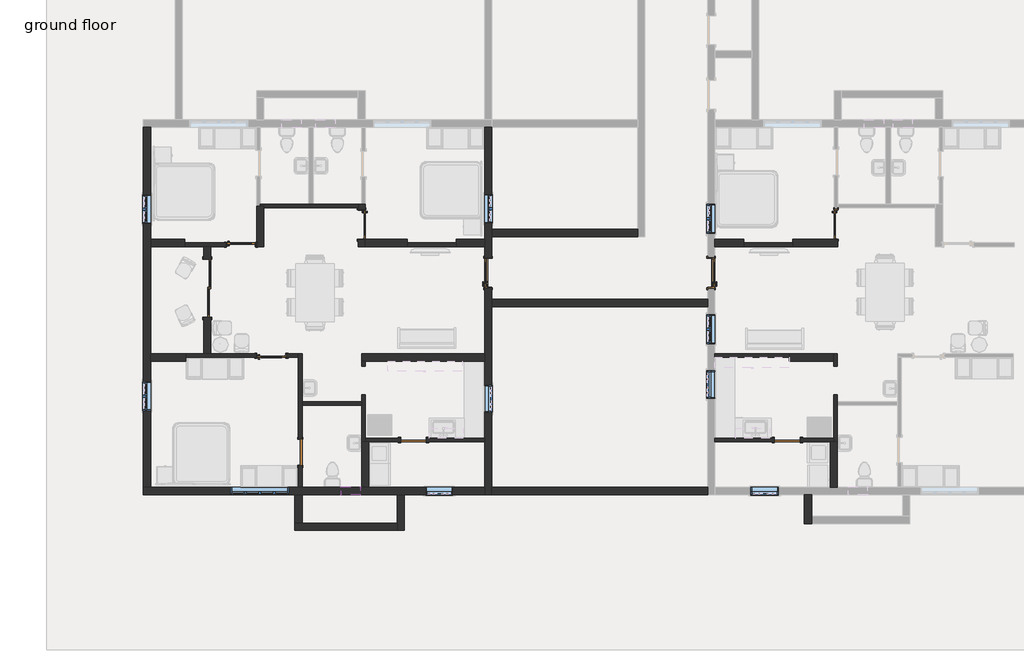
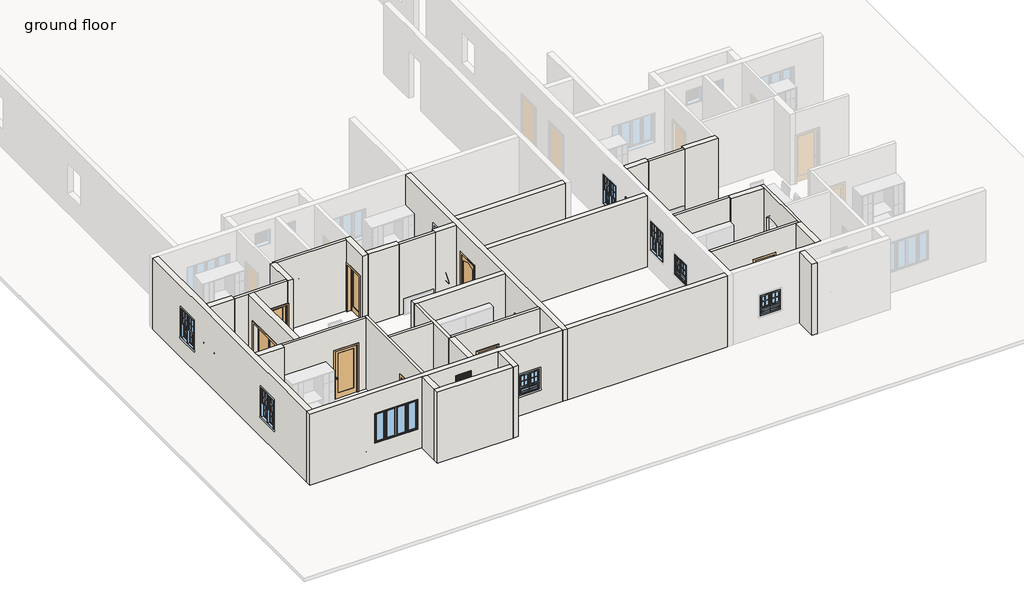
# One storey, part 1 of 16: 35 walls, 11 windows, 10 doors.
"""IFC4 building model written with IfcOpenShell, lengths in millimetres."""

from ifc_helpers import new_model, si_unit, point, frame, origin, place, context, project, spatial, polyline, ellipse_curve, trimmed, outline, extrude, faceted_brep, transform, mapped, element, save
from ifc_brep_helpers import plane_surface, extruded_surface, advanced_brep
from components import door_fe8ae985, door_f079f64e, door_d4d75d1e, door_a3feeac7, door_3c6ab76a, door_3b97b8e7, door_38851409, door_d141acb4, window_ced37e8f, window_5487fb6d, window_f2d8fef0, window_45970670

model = new_model("IFC4")

# Units and contexts
model_context = context("Model", 3, world=origin())
ifc_project = project(units=[si_unit("LENGTHUNIT", "METRE", prefix="MILLI")], contexts=[model_context])

# Site, building, storey
site = spatial("IfcSite", under=ifc_project)
building = spatial("IfcBuilding", under=site)
storey = spatial("IfcBuildingStorey", under=building, Name="ground floor", Elevation=609.6)

# Doors
placement = place(None, origin())
door_shape = door_fe8ae985(model_context)
element("IfcDoor", 1, ObjectType="36\" x 84\"", at=placement, inside=storey, context=model_context, shape_type="MappedRepresentation", body=[
    mapped(door_shape, transform((52422.151243, -18346.451256, 609.6), x_axis=(0.0, -1.0, 0.0), y_axis=(1.0, 0.0, 0.0), z_axis=(0.0, 0.0, 1.0))),
])
door_2_shape = door_f079f64e(model_context)
element("IfcDoor", 2, ObjectType="36\" x 84\"", at=placement, inside=storey, context=model_context, shape_type="MappedRepresentation", body=[
    mapped(door_2_shape, transform((59474.0062819, -18346.451256, 609.6), x_axis=(0.0, -1.0, 0.0), y_axis=(1.0, 0.0, 0.0), z_axis=(0.0, 0.0, 1.0))),
])
door_3_shape = door_d4d75d1e(model_context)
element("IfcDoor", 3, ObjectType="Door-Double-Sliding : 72\" x 84\"", at=placement, inside=storey, context=model_context, shape_type="MappedRepresentation", body=[
    mapped(door_3_shape, transform((43421.026243, -18827.9865909, 609.6), x_axis=(0.0, -1.0, 0.0), y_axis=(1.0, 0.0, 0.0), z_axis=(0.0, 0.0, 1.0))),
])
door_4_shape = door_a3feeac7(model_context)
element("IfcDoor", 4, ObjectType="Door-Interior-Single-1_Panel-Wood : 36\" x 84\"", at=placement, inside=storey, context=model_context, shape_type="MappedRepresentation", body=[
    mapped(door_4_shape, transform((45573.676243, -20964.7615909, 609.6), x_axis=(1.0, 0.0, 0.0), y_axis=(0.0, 1.0, 0.0), z_axis=(0.0, 0.0, 1.0))),
])
element("IfcDoor", 5, ObjectType="Door-Interior-Single-1_Panel-Wood : 36\" x 84\"", at=placement, inside=storey, context=model_context, shape_type="MappedRepresentation", body=[
    mapped(door_4_shape, transform((63411.0062819, -16818.2115909, 609.6), x_axis=(0.0, -1.0, 0.0), y_axis=(1.0, 0.0, 0.0), z_axis=(0.0, 0.0, 1.0))),
])
door_5_shape = door_3c6ab76a(model_context)
element("IfcDoor", 6, ObjectType="Door-Interior-Single-1_Panel-Wood : 36\" x 84\"", at=placement, inside=storey, context=model_context, shape_type="MappedRepresentation", body=[
    mapped(door_5_shape, transform((44614.826243, -17453.2115909, 609.6), x_axis=(1.0, 0.0, 0.0), y_axis=(0.0, 1.0, 0.0), z_axis=(0.0, 0.0, 1.0))),
])
door_6_shape = door_3b97b8e7(model_context)
element("IfcDoor", 7, ObjectType="Door-Interior-Single-1_Panel-Wood : 36\" x 84\"", at=placement, inside=storey, context=model_context, shape_type="MappedRepresentation", body=[
    mapped(door_6_shape, transform((48432.1907505, -16818.2115909, 609.6), x_axis=(0.0, -1.0, 0.0), y_axis=(1.0, 0.0, 0.0), z_axis=(0.0, 0.0, 1.0))),
])
door_7_shape = door_38851409(model_context)
element("IfcDoor", 8, ObjectType="Single-Flush : 32\" x 84\"", at=placement, inside=storey, context=model_context, shape_type="MappedRepresentation", body=[
    mapped(door_7_shape, transform((61877.4812819, -23628.4658586, 609.6), x_axis=(1.0, 0.0, 0.0), y_axis=(0.0, 1.0, 0.0), z_axis=(0.0, 0.0, 1.0))),
])
element("IfcDoor", 9, ObjectType="Single-Flush : 32\" x 84\"", at=placement, inside=storey, context=model_context, shape_type="MappedRepresentation", body=[
    mapped(door_7_shape, transform((46488.076243, -24015.9365909, 609.6), x_axis=(0.0, 1.0, 0.0), y_axis=(-1.0, 0.0, 0.0), z_axis=(0.0, 0.0, 1.0))),
])
door_8_shape = door_d141acb4(model_context)
element("IfcDoor", 10, ObjectType="Single-Flush : 32\" x 84\"", at=placement, inside=storey, context=model_context, shape_type="MappedRepresentation", body=[
    mapped(door_8_shape, transform((50063.126243, -23628.5865909, 609.6), x_axis=(-1.0, 0.0, 0.0), y_axis=(0.0, -1.0, 0.0), z_axis=(0.0, 0.0, 1.0))),
])

# Walls
element("IfcWall", 11, ObjectType="Generic - 4.5\"", at=placement, inside=storey, context=model_context, shape_type="Brep", body=[
    faceted_brep([(46545.226243, -23609.5365909, 2743.2), (46545.226243, -23609.5365909, 609.6), (46545.226243, -22530.0365909, 609.6), (46545.226243, -22415.7365909, 609.6), (46545.226243, -20904.4365909, 609.6), (46545.226243, -20904.4365909, 3810.0), (46545.226243, -22415.7365909, 3810.0), (46545.226243, -22530.0365909, 3810.0), (46545.226243, -25120.8365909, 3810.0), (46545.226243, -25120.8365909, 609.6), (46545.226243, -24422.3365909, 609.6), (46545.226243, -24422.3365909, 2743.2), (46430.926243, -20904.4365909, 609.6), (46430.926243, -21018.7365909, 609.6), (46430.926243, -23609.5365909, 609.6), (46430.926243, -23609.5365909, 2743.2), (46430.926243, -24422.3365909, 2743.2), (46430.926243, -24422.3365909, 609.6), (46430.926243, -25120.8365909, 609.6), (46430.926243, -25120.8365909, 3810.0), (46430.926243, -21018.7365909, 3810.0), (46430.926243, -20904.4365909, 3810.0)], [[[0, 1, 2, 3, 4, 5, 6, 7, 8, 9, 10, 11]], [[12, 13, 14, 15, 16, 17, 18, 19, 20, 21]], [[10, 9, 18, 17]], [[4, 3, 2, 1, 14, 13, 12]], [[8, 7, 6, 5, 21, 20, 19]], [[9, 8, 19, 18]], [[5, 4, 12, 21]], [[15, 14, 1, 0]], [[16, 15, 0, 11]], [[17, 16, 11, 10]]]),
])
element("IfcWall", 12, ObjectType="Generic - 4.5\"", at=placement, inside=storey, context=model_context, shape_type="Brep", body=[
    faceted_brep([(42874.926243, -20904.4365909, 609.6), (42874.926243, -20904.4365909, 3810.0), (43433.726243, -20904.4365909, 3810.0), (43662.326243, -20904.4365909, 3810.0), (46430.926243, -20904.4365909, 3810.0), (46430.926243, -20904.4365909, 609.6), (46056.276243, -20904.4365909, 609.6), (46056.276243, -20904.4365909, 2768.6), (45091.076243, -20904.4365909, 2768.6), (45091.076243, -20904.4365909, 609.6), (43662.326243, -20904.4365909, 609.6), (43433.726243, -20904.4365909, 609.6), (42874.926243, -21018.7365909, 3810.0), (42874.926243, -21018.7365909, 609.6), (45091.076243, -21018.7365909, 609.6), (45091.076243, -21018.7365909, 2768.6), (46056.276243, -21018.7365909, 2768.6), (46056.276243, -21018.7365909, 609.6), (46430.926243, -21018.7365909, 609.6), (46430.926243, -21018.7365909, 3810.0)], [[[0, 1, 2, 3, 4, 5, 6, 7, 8, 9, 10, 11]], [[12, 13, 14, 15, 16, 17, 18, 19]], [[5, 18, 17, 6]], [[13, 0, 11, 10, 9, 14]], [[1, 0, 13, 12]], [[4, 3, 2, 1, 12, 19]], [[5, 4, 19, 18]], [[16, 7, 6, 17]], [[7, 16, 15, 8]], [[8, 15, 14, 9]]]),
])
element("IfcWall", 13, ObjectType="Generic - 4.5\"", at=placement, inside=storey, context=model_context, shape_type="SweptSolid", body=[
    extrude(outline(polyline([(48424.826243, -22530.0365909), (46545.226243, -22530.0365909), (46545.226243, -22415.7365909), (48424.826243, -22415.7365909), (48424.826243, -22530.0365909)])), frame((0.0, 0.0, 609.6), z_axis=(0.0, 0.0, 1.0), x_axis=(1.0, 0.0, 0.0)), (0.0, 0.0, 1.0), 3200.4),
])
element("IfcWall", 14, ObjectType="Generic - 4.5\"", at=placement, inside=storey, context=model_context, shape_type="AdvancedBrep", body=[
    advanced_brep(
    [(48424.826243, -21133.0365909, 609.6), (48424.826243, -21288.6115909, 609.6), (48424.826243, -21288.6115909, 2540.0), (48424.826243, -22203.0115909, 2540.0), (48424.826243, -22203.0115909, 609.6), (48424.826243, -22415.7365909, 609.6), (48424.826243, -22530.0365909, 609.6), (48424.826243, -23685.7365909, 609.6), (48424.826243, -23685.7365909, 3810.0), (48424.826243, -22530.0365909, 3810.0), (48424.826243, -22415.7365909, 3810.0), (48424.826243, -21133.0365909, 3810.0), (48539.126243, -21288.6115909, 2540.0), (48539.126243, -21288.6115909, 609.6), (48539.126243, -21133.0365909, 609.6), (48539.126243, -21133.0365909, 3810.0), (48539.126243, -23571.4365909, 3810.0), (48539.126243, -23685.7365909, 3810.0), (48539.126243, -23685.7365909, 609.6), (48539.126243, -23571.4365909, 609.6), (48539.126243, -22203.0115909, 609.6), (48539.126243, -22203.0115909, 2540.0)],
    [
        (0, 1),
        (1, 2),
        (2, 3, ellipse_curve(frame((48424.826243, -21745.8115909, 2540.0), z_axis=(1.0, 0.0, 0.0), x_axis=(0.0, 1.0, 0.0)), 457.2, 203.2)),
        (3, 4),
        (4, 5),
        (5, 6),
        (6, 7),
        (7, 8),
        (8, 9),
        (9, 10),
        (10, 11),
        (11, 0),
        (12, 13),
        (13, 14),
        (14, 15),
        (15, 16),
        (16, 17),
        (17, 18),
        (18, 19),
        (19, 20),
        (20, 21),
        (21, 12, ellipse_curve(frame((48539.126243, -21745.8115909, 2540.0), z_axis=(-1.0, 0.0, 0.0), x_axis=(0.0, 1.0, 0.0)), 457.2, 203.2)),
        (13, 1),
        (0, 14),
        (18, 7),
        (4, 20),
        (8, 17),
        (15, 11),
        (2, 12),
        (21, 3),
    ],
    [
        plane_surface(frame((48424.826243, -22415.7365909, 609.6), z_axis=(-1.0, 0.0, 0.0), x_axis=(0.0, -1.0, 0.0))),
        plane_surface(frame((48539.126243, -22415.7365909, 609.6), z_axis=(1.0, 0.0, 0.0), x_axis=(0.0, 1.0, 0.0))),
        plane_surface(frame((48424.826243, -21018.7365909, 609.6), z_axis=(0.0, 0.0, -1.0), x_axis=(1.0, 0.0, 0.0))),
        plane_surface(frame((48424.826243, -23628.5865909, 3810.0), z_axis=(0.0, 0.0, 1.0), x_axis=(1.0, 0.0, 0.0))),
        plane_surface(frame((48541.8036793, -23685.7365909, 609.6), z_axis=(0.0, -1.0, 0.0), x_axis=(1.0, 0.0, 0.0))),
        plane_surface(frame((48424.826243, -21133.0365909, 609.6), z_axis=(0.0, 1.0, 0.0), x_axis=(1.0, 0.0, 0.0))),
        extruded_surface(trimmed(ellipse_curve(frame((48653.426243, -21745.8115909, 2540.0), z_axis=(1.0, 0.0, 0.0), x_axis=(0.0, 1.0, 0.0)), 457.2, 203.2), [point((48653.426243, -21288.6115909, 2540.0))], [point((48653.426243, -22203.0115909, 2540.0))], True, "CARTESIAN"), (-114.30000000000291, 0.0, 0.0), 114.30000000000291),
        plane_surface(frame((48424.826243, -22203.0115909, 2540.0), z_axis=(0.0, 1.0, 0.0), x_axis=(1.0, 0.0, 0.0))),
        plane_surface(frame((48424.826243, -21288.6115909, 609.6), z_axis=(0.0, -1.0, 0.0), x_axis=(1.0, 0.0, 0.0))),
    ],
    [
        (0, [[1, 2, 3, 4, 5, 6, 7, 8, 9, 10, 11, 12]]),
        (1, [[13, 14, 15, 16, 17, 18, 19, 20, 21, 22]]),
        (2, [[-14, 23, -1, 24]]),
        (2, [[-20, -19, 25, -7, -6, -5, 26]]),
        (3, [[-11, -10, -9, 27, -17, -16, 28]]),
        (4, [[-8, -25, -18, -27]]),
        (5, [[-12, -28, -15, -24]]),
        (6, [[-3, 29, -22, 30]]),
        (7, [[-4, -30, -21, -26]]),
        (8, [[-2, -23, -13, -29]]),
    ],
),
])
element("IfcWall", 15, ObjectType="Generic - 4.5\"", at=placement, inside=storey, context=model_context, shape_type="Brep", body=[
    faceted_brep([(48539.126243, -23685.7365909, 609.6), (48653.426243, -23685.7365909, 609.6), (49656.726243, -23685.7365909, 609.6), (49656.726243, -23685.7365909, 2743.2), (50469.526243, -23685.7365909, 2743.2), (50469.526243, -23685.7365909, 609.6), (52311.026243, -23685.7365909, 609.6), (52311.026243, -23685.7365909, 3810.0), (48653.426243, -23685.7365909, 3810.0), (48539.126243, -23685.7365909, 3810.0), (49656.726243, -23571.4365909, 2743.2), (49656.726243, -23571.4365909, 609.6), (48539.126243, -23571.4365909, 609.6), (48539.126243, -23571.4365909, 3810.0), (52311.026243, -23571.4365909, 3810.0), (52311.026243, -23571.4365909, 609.6), (50469.526243, -23571.4365909, 609.6), (50469.526243, -23571.4365909, 2743.2)], [[[0, 1, 2, 3, 4, 5, 6, 7, 8, 9]], [[10, 11, 12, 13, 14, 15, 16, 17]], [[16, 15, 6, 5]], [[12, 11, 2, 1, 0]], [[9, 8, 7, 14, 13]], [[0, 9, 13, 12]], [[7, 6, 15, 14]], [[3, 2, 11, 10]], [[4, 3, 10, 17]], [[5, 4, 17, 16]]]),
])
element("IfcWall", 16, ObjectType="Generic - 4.5\"", at=placement, inside=storey, context=model_context, shape_type="SweptSolid", body=[
    extrude(outline(polyline([(51409.326243, -17513.5365909), (49864.1157505, -17513.5365909), (49864.1157505, -17399.2365909), (51409.326243, -17399.2365909), (51409.326243, -17513.5365909)])), frame((0.0, 0.0, 609.6), z_axis=(0.0, 0.0, 1.0), x_axis=(1.0, 0.0, 0.0)), (0.0, 0.0, 1.0), 3200.4),
])
element("IfcWall", 17, ObjectType="Generic - 4.5\"", at=placement, inside=storey, context=model_context, shape_type="Brep", body=[
    faceted_brep([(45110.126243, -17513.5365909, 3810.0), (43662.326243, -17513.5365909, 3810.0), (43433.726243, -17513.5365909, 3810.0), (42841.8030199, -17513.5365909, 3810.0), (42841.8030199, -17513.5365909, 609.6), (43433.726243, -17513.5365909, 609.6), (43662.326243, -17513.5365909, 609.6), (44132.226243, -17513.5365909, 609.6), (44132.226243, -17513.5365909, 2768.6), (45097.426243, -17513.5365909, 2768.6), (45097.426243, -17513.5365909, 609.6), (45110.126243, -17513.5365909, 609.6), (42841.8030199, -17399.2365909, 3810.0), (45110.126243, -17399.2365909, 3810.0), (45110.126243, -17399.2365909, 609.6), (45097.426243, -17399.2365909, 609.6), (45097.426243, -17399.2365909, 2768.6), (44132.226243, -17399.2365909, 2768.6), (44132.226243, -17399.2365909, 609.6), (42841.8030199, -17399.2365909, 609.6)], [[[0, 1, 2, 3, 4, 5, 6, 7, 8, 9, 10, 11]], [[12, 13, 14, 15, 16, 17, 18, 19]], [[4, 19, 18, 7, 6, 5]], [[14, 11, 10, 15]], [[3, 2, 1, 0, 13, 12]], [[4, 3, 12, 19]], [[0, 11, 14, 13]], [[9, 16, 15, 10]], [[16, 9, 8, 17]], [[17, 8, 7, 18]]]),
])
element("IfcWall", 18, ObjectType="Generic - 4.5\"", at=placement, inside=storey, context=model_context, shape_type="Brep", body=[
    faceted_brep([(45338.726243, -16294.3365909, 609.6), (48314.7157505, -16294.3365909, 609.6), (48314.7157505, -16294.3365909, 3810.0), (45338.726243, -16294.3365909, 3810.0), (45227.7264835, -16180.0365909, 609.6), (45227.7264835, -16180.0365909, 3810.0), (46748.426243, -16180.0365909, 3810.0), (46900.826243, -16180.0365909, 3810.0), (48314.7157505, -16180.0365909, 3810.0), (48314.7157505, -16180.0365909, 609.6), (46900.826243, -16180.0365909, 609.6), (46748.426243, -16180.0365909, 609.6), (45338.726243, -16237.1865909, 609.6), (45227.7264835, -16237.1865909, 609.6), (45227.7264835, -16237.1865909, 3810.0), (45338.726243, -16237.1865909, 3810.0)], [[[0, 1, 2, 3]], [[4, 5, 6, 7, 8, 9, 10, 11]], [[1, 0, 12, 13, 4, 11, 10, 9]], [[3, 2, 8, 7, 6, 5, 14, 15]], [[2, 1, 9, 8]], [[0, 3, 15, 12]], [[15, 14, 13, 12]], [[14, 5, 4, 13]]]),
])
element("IfcWall", 19, ObjectType="Generic - 4.5\"", at=placement, inside=storey, context=model_context, shape_type="AdvancedBrep", body=[
    advanced_brep(
    [(63344.3312819, -22202.0724681, 2540.0), (63344.3312819, -22202.0724681, 609.6), (63344.3312819, -23571.3158586, 609.6), (63344.3312819, -23685.6158586, 609.6), (63344.3312819, -23685.6158586, 3810.0), (63344.3312819, -23571.3158586, 3810.0), (63344.3312819, -21132.9158586, 3810.0), (63344.3312819, -20904.3158586, 3810.0), (63344.3312819, -20904.3158586, 609.6), (63344.3312819, -21132.9158586, 609.6), (63344.3312819, -21287.6724681, 609.6), (63344.3312819, -21287.6724681, 2540.0), (63458.6312819, -23685.6158586, 609.6), (63458.6312819, -22528.2790776, 609.6), (63458.6312819, -22413.9790776, 609.6), (63458.6312819, -22202.0724681, 609.6), (63458.6312819, -22202.0724681, 2540.0), (63458.6312819, -21287.6724681, 2540.0), (63458.6312819, -21287.6724681, 609.6), (63458.6312819, -20904.3158586, 609.6), (63458.6312819, -20904.3158586, 3810.0), (63458.6312819, -22413.9790776, 3810.0), (63458.6312819, -22528.2790776, 3810.0), (63458.6312819, -23685.6158586, 3810.0)],
    [
        (0, 1),
        (1, 2),
        (2, 3),
        (3, 4),
        (4, 5),
        (5, 6),
        (6, 7),
        (7, 8),
        (8, 9),
        (9, 10),
        (10, 11),
        (11, 0, ellipse_curve(frame((63344.3312819, -21744.8724681, 2540.0), z_axis=(1.0, 0.0, 0.0), x_axis=(0.0, -1.0, 0.0)), 457.2, 203.2)),
        (12, 13),
        (13, 14),
        (14, 15),
        (15, 16),
        (16, 17, ellipse_curve(frame((63458.6312819, -21744.8724681, 2540.0), z_axis=(-1.0, 0.0, 0.0), x_axis=(0.0, -1.0, 0.0)), 457.2, 203.2)),
        (17, 18),
        (18, 19),
        (19, 20),
        (20, 21),
        (21, 22),
        (22, 23),
        (23, 12),
        (8, 19),
        (18, 10),
        (1, 15),
        (12, 3),
        (4, 23),
        (20, 7),
        (16, 0),
        (11, 17),
    ],
    [
        plane_surface(frame((63344.3312819, -21132.9158586, 609.6), z_axis=(-1.0, 0.0, 0.0), x_axis=(0.0, -1.0, 0.0))),
        plane_surface(frame((63458.6312819, -21132.9158586, 609.6), z_axis=(1.0, 0.0, 0.0), x_axis=(0.0, 1.0, 0.0))),
        plane_surface(frame((63344.3312819, -21018.6158586, 609.6), z_axis=(0.0, 0.0, -1.0), x_axis=(1.0, 0.0, 0.0))),
        plane_surface(frame((63344.3312819, -23628.4658586, 3810.0), z_axis=(0.0, 0.0, 1.0), x_axis=(1.0, 0.0, 0.0))),
        plane_surface(frame((63444.0943847, -23685.6158586, 609.6), z_axis=(0.0, -1.0, 0.0), x_axis=(1.0, 0.0, 0.0))),
        plane_surface(frame((63433.2312819, -20904.3158586, 609.6), z_axis=(0.0, 1.0, 0.0), x_axis=(-1.0, 0.0, 0.0))),
        extruded_surface(trimmed(ellipse_curve(frame((63230.0312819, -21744.8724681, 2540.0), z_axis=(-1.0, 0.0, 0.0), x_axis=(0.0, -1.0, 0.0)), 457.2, 203.2), [point((63230.0312819, -22202.0724681, 2540.0))], [point((63230.0312819, -21287.6724681, 2540.0))], True, "CARTESIAN"), (114.29999999999563, 0.0, 0.0), 114.29999999999563),
        plane_surface(frame((63458.6312819, -21287.6724681, 2540.0), z_axis=(0.0, -1.0, 0.0), x_axis=(-1.0, 0.0, 0.0))),
        plane_surface(frame((63458.6312819, -22202.0724681, 609.6), z_axis=(0.0, 1.0, 0.0), x_axis=(-1.0, 0.0, 0.0))),
    ],
    [
        (0, [[1, 2, 3, 4, 5, 6, 7, 8, 9, 10, 11, 12]]),
        (1, [[13, 14, 15, 16, 17, 18, 19, 20, 21, 22, 23, 24]]),
        (2, [[-10, -9, 25, -19, 26]]),
        (2, [[-3, -2, 27, -15, -14, -13, 28]]),
        (3, [[-7, -6, -5, 29, -23, -22, -21, 30]]),
        (4, [[-4, -28, -24, -29]]),
        (5, [[-8, -30, -20, -25]]),
        (6, [[-17, 31, -12, 32]]),
        (7, [[-18, -32, -11, -26]]),
        (8, [[-16, -27, -1, -31]]),
    ],
),
])
element("IfcWall", 20, ObjectType="Generic - 4.5\"", at=placement, inside=storey, context=model_context, shape_type="Brep", body=[
    faceted_brep([(63344.3312819, -23571.3158586, 609.6), (62283.8812819, -23571.3158586, 609.6), (62283.8812819, -23571.3158586, 2743.2), (61471.0812819, -23571.3158586, 2743.2), (61471.0812819, -23571.3158586, 609.6), (59585.1312819, -23571.3158586, 609.6), (59585.1312819, -23571.3158586, 3810.0), (63344.3312819, -23571.3158586, 3810.0), (62283.8812819, -23685.6158586, 2743.2), (62283.8812819, -23685.6158586, 609.6), (63230.0312819, -23685.6158586, 609.6), (63344.3312819, -23685.6158586, 609.6), (63344.3312819, -23685.6158586, 3810.0), (63230.0312819, -23685.6158586, 3810.0), (59585.1312819, -23685.6158586, 3810.0), (59585.1312819, -23685.6158586, 609.6), (61471.0812819, -23685.6158586, 609.6), (61471.0812819, -23685.6158586, 2743.2)], [[[0, 1, 2, 3, 4, 5, 6, 7]], [[8, 9, 10, 11, 12, 13, 14, 15, 16, 17]], [[16, 15, 5, 4]], [[11, 10, 9, 1, 0]], [[7, 6, 14, 13, 12]], [[0, 7, 12, 11]], [[6, 5, 15, 14]], [[2, 1, 9, 8]], [[3, 2, 8, 17]], [[4, 3, 17, 16]]]),
])
element("IfcWall", 21, ObjectType="Generic - 4.5\"", at=placement, inside=storey, context=model_context, shape_type="SweptSolid", body=[
    extrude(outline(polyline([(61947.3312819, -21018.6158586), (59585.1312819, -21018.6158586), (59585.1312819, -20904.3158586), (61947.3312819, -20904.3158586), (61947.3312819, -21018.6158586)])), frame((0.0, 0.0, 609.6), z_axis=(0.0, 0.0, 1.0), x_axis=(1.0, 0.0, 0.0)), (0.0, 0.0, 1.0), 3200.4),
])
element("IfcWall", 22, ObjectType="Generic - 4.5\"", at=placement, inside=storey, context=model_context, shape_type="SweptSolid", body=[
    extrude(outline(polyline([(62052.7675141, -17513.5365909), (60506.3427006, -17513.5365909), (60506.3427006, -17399.2365909), (62052.7675141, -17399.2365909), (62052.7675141, -17513.5365909)])), frame((0.0, 0.0, 609.6), z_axis=(0.0, 0.0, 1.0), x_axis=(1.0, 0.0, 0.0)), (0.0, 0.0, 1.0), 3200.4),
])
element("IfcWall", 23, ObjectType="Generic - 9\"", at=placement, inside=storey, context=model_context, shape_type="Brep", body=[
    faceted_brep([(52311.026243, -25349.4365909, 3810.0), (52311.026243, -25120.8365909, 3810.0), (52311.026243, -23685.7365909, 3810.0), (52311.026243, -23571.4365909, 3810.0), (52311.026243, -21133.0365909, 3810.0), (52311.026243, -20904.4365909, 3810.0), (52311.026243, -17513.5365909, 3810.0), (52311.026243, -17284.9365909, 3810.0), (52311.026243, -13741.6365909, 3810.0), (52311.026243, -13741.6365909, 609.6), (52311.026243, -17284.9365909, 609.6), (52311.026243, -17513.5365909, 609.6), (52311.026243, -17863.851256, 609.6), (52311.026243, -17863.851256, 2768.6), (52311.026243, -18829.051256, 2768.6), (52311.026243, -18829.051256, 609.6), (52311.026243, -20904.4365909, 609.6), (52311.026243, -21133.0365909, 609.6), (52311.026243, -23571.4365909, 609.6), (52311.026243, -23685.7365909, 609.6), (52311.026243, -25120.8365909, 609.6), (52311.026243, -25349.4365909, 609.6), (52311.026243, -15864.6659211, 2844.8), (52311.026243, -16779.0659211, 2844.8), (52311.026243, -16779.0659211, 1524.0), (52311.026243, -15864.6659211, 1524.0), (52311.026243, -22755.4615909, 2438.4), (52311.026243, -22755.4615909, 1524.0), (52311.026243, -21891.8615909, 1524.0), (52311.026243, -21891.8615909, 2438.4), (52539.626243, -13741.6365909, 3810.0), (52539.626243, -16969.5659211, 3810.0), (52539.626243, -17198.1659211, 3810.0), (52539.626243, -19179.3659211, 3810.0), (52539.626243, -19407.9659211, 3810.0), (52539.626243, -25120.8365909, 3810.0), (52539.626243, -25349.4365909, 3810.0), (52539.626243, -25349.4365909, 609.6), (52539.626243, -25120.8365909, 609.6), (52539.626243, -19407.9659211, 609.6), (52539.626243, -19179.3659211, 609.6), (52539.626243, -18829.051256, 609.6), (52539.626243, -18829.051256, 2768.6), (52539.626243, -17863.851256, 2768.6), (52539.626243, -17863.851256, 609.6), (52539.626243, -17198.1659211, 609.6), (52539.626243, -16969.5659211, 609.6), (52539.626243, -13741.6365909, 609.6), (52539.626243, -15864.6659211, 2844.8), (52539.626243, -15864.6659211, 1524.0), (52539.626243, -16779.0659211, 1524.0), (52539.626243, -16779.0659211, 2844.8), (52539.626243, -22755.4615909, 2438.4), (52539.626243, -21891.8615909, 2438.4), (52539.626243, -21891.8615909, 1524.0), (52539.626243, -22755.4615909, 1524.0)], [[[0, 1, 2, 3, 4, 5, 6, 7, 8, 9, 10, 11, 12, 13, 14, 15, 16, 17, 18, 19, 20, 21], [22, 23, 24, 25], [26, 27, 28, 29]], [[30, 31, 32, 33, 34, 35, 36, 37, 38, 39, 40, 41, 42, 43, 44, 45, 46, 47], [48, 49, 50, 51], [52, 53, 54, 55]], [[9, 47, 46, 45, 44, 12, 11, 10]], [[37, 21, 20, 19, 18, 17, 16, 15, 41, 40, 39, 38]], [[8, 7, 6, 5, 4, 3, 2, 1, 0, 36, 35, 34, 33, 32, 31, 30]], [[9, 8, 30, 47]], [[0, 21, 37, 36]], [[14, 42, 41, 15]], [[42, 14, 13, 43]], [[43, 13, 12, 44]], [[49, 48, 22, 25]], [[50, 49, 25, 24]], [[51, 50, 24, 23]], [[48, 51, 23, 22]], [[27, 26, 52, 55]], [[28, 27, 55, 54]], [[29, 28, 54, 53]], [[26, 29, 53, 52]]]),
])
element("IfcWall", 24, ObjectType="Generic - 9\"", at=placement, inside=storey, context=model_context, shape_type="Brep", body=[
    faceted_brep([(52311.026243, -25120.8365909, 609.6), (48653.426243, -25120.8365909, 609.6), (48424.826243, -25120.8365909, 609.6), (46545.226243, -25120.8365909, 609.6), (46430.926243, -25120.8365909, 609.6), (41757.326243, -25120.8365909, 609.6), (41528.726243, -25120.8365909, 609.6), (41528.726243, -25120.8365909, 3810.0), (41757.326243, -25120.8365909, 3810.0), (46430.926243, -25120.8365909, 3810.0), (46545.226243, -25120.8365909, 3810.0), (48424.826243, -25120.8365909, 3810.0), (48653.426243, -25120.8365909, 3810.0), (52311.026243, -25120.8365909, 3810.0), (44295.434231, -25120.8365909, 2870.2), (44295.434231, -25120.8365909, 1524.0), (46124.234231, -25120.8365909, 1524.0), (46124.234231, -25120.8365909, 2870.2), (50449.707768, -25120.8365909, 2438.4), (50449.707768, -25120.8365909, 1524.0), (51313.307768, -25120.8365909, 1524.0), (51313.307768, -25120.8365909, 2438.4), (48386.726243, -25120.8365909, 3352.8), (47777.126243, -25120.8365909, 3352.8), (47777.126243, -25120.8365909, 2743.2), (48386.726243, -25120.8365909, 2743.2), (52311.026243, -25349.4365909, 609.6), (52311.026243, -25349.4365909, 3810.0), (49776.607768, -25349.4365909, 3810.0), (49548.007768, -25349.4365909, 3810.0), (46543.334231, -25349.4365909, 3810.0), (46314.734231, -25349.4365909, 3810.0), (41528.726243, -25349.4365909, 3810.0), (41528.726243, -25349.4365909, 609.6), (46314.734231, -25349.4365909, 609.6), (46543.334231, -25349.4365909, 609.6), (49548.007768, -25349.4365909, 609.6), (49776.607768, -25349.4365909, 609.6), (44295.434231, -25349.4365909, 2870.2), (46124.234231, -25349.4365909, 2870.2), (46124.234231, -25349.4365909, 1524.0), (44295.434231, -25349.4365909, 1524.0), (50449.707768, -25349.4365909, 2438.4), (51313.307768, -25349.4365909, 2438.4), (51313.307768, -25349.4365909, 1524.0), (50449.707768, -25349.4365909, 1524.0), (48386.726243, -25349.4365909, 3352.8), (48386.726243, -25349.4365909, 2743.2), (47777.126243, -25349.4365909, 2743.2), (47777.126243, -25349.4365909, 3352.8)], [[[0, 1, 2, 3, 4, 5, 6, 7, 8, 9, 10, 11, 12, 13], [14, 15, 16, 17], [18, 19, 20, 21], [22, 23, 24, 25]], [[26, 27, 28, 29, 30, 31, 32, 33, 34, 35, 36, 37], [38, 39, 40, 41], [42, 43, 44, 45], [46, 47, 48, 49]], [[6, 5, 4, 3, 2, 1, 0, 26, 37, 36, 35, 34, 33]], [[13, 12, 11, 10, 9, 8, 7, 32, 31, 30, 29, 28, 27]], [[0, 13, 27, 26]], [[7, 6, 33, 32]], [[15, 14, 38, 41]], [[16, 15, 41, 40]], [[17, 16, 40, 39]], [[14, 17, 39, 38]], [[19, 18, 42, 45]], [[20, 19, 45, 44]], [[21, 20, 44, 43]], [[18, 21, 43, 42]], [[47, 46, 22, 25]], [[48, 47, 25, 24]], [[49, 48, 24, 23]], [[46, 49, 23, 22]]]),
])
element("IfcWall", 25, ObjectType="Generic - 9\"", at=placement, inside=storey, context=model_context, shape_type="Brep", body=[
    faceted_brep([(41757.326243, -25120.8365909, 609.6), (41757.326243, -21133.0365909, 609.6), (41757.326243, -20904.4365909, 609.6), (41757.326243, -17513.5365909, 609.6), (41757.326243, -17284.9365909, 609.6), (41757.326243, -13741.6365909, 609.6), (41757.326243, -13741.6365909, 3810.0), (41757.326243, -17284.9365909, 3810.0), (41757.326243, -17513.5365909, 3810.0), (41757.326243, -20904.4365909, 3810.0), (41757.326243, -21133.0365909, 3810.0), (41757.326243, -25120.8365909, 3810.0), (41757.326243, -22695.1365909, 2844.8), (41757.326243, -21780.7365909, 2844.8), (41757.326243, -21780.7365909, 1524.0), (41757.326243, -22695.1365909, 1524.0), (41757.326243, -16789.6365909, 2844.8), (41757.326243, -15875.2365909, 2844.8), (41757.326243, -15875.2365909, 1524.0), (41757.326243, -16789.6365909, 1524.0), (41528.726243, -25120.8365909, 609.6), (41528.726243, -25120.8365909, 3810.0), (41528.726243, -13741.6365909, 3810.0), (41528.726243, -13741.6365909, 609.6), (41528.726243, -22695.1365909, 2844.8), (41528.726243, -22695.1365909, 1524.0), (41528.726243, -21780.7365909, 1524.0), (41528.726243, -21780.7365909, 2844.8), (41528.726243, -16789.6365909, 2844.8), (41528.726243, -16789.6365909, 1524.0), (41528.726243, -15875.2365909, 1524.0), (41528.726243, -15875.2365909, 2844.8)], [[[0, 1, 2, 3, 4, 5, 6, 7, 8, 9, 10, 11], [12, 13, 14, 15], [16, 17, 18, 19]], [[20, 21, 22, 23], [24, 25, 26, 27], [28, 29, 30, 31]], [[5, 4, 3, 2, 1, 0, 20, 23]], [[11, 10, 9, 8, 7, 6, 22, 21]], [[6, 5, 23, 22]], [[0, 11, 21, 20]], [[25, 24, 12, 15]], [[26, 25, 15, 14]], [[27, 26, 14, 13]], [[24, 27, 13, 12]], [[29, 28, 16, 19]], [[30, 29, 19, 18]], [[31, 30, 18, 17]], [[28, 31, 17, 16]]]),
])
element("IfcWall", 26, ObjectType="Generic - 9\"", at=placement, inside=storey, context=model_context, shape_type="Brep", body=[
    faceted_brep([(41757.326243, -17513.5365909, 609.6), (42841.8030199, -17513.5365909, 609.6), (42841.8030199, -17513.5365909, 3810.0), (41757.326243, -17513.5365909, 3810.0), (41757.326243, -17284.9365909, 609.6), (41757.326243, -17284.9365909, 3810.0), (42841.8030199, -17284.9365909, 3810.0), (42841.8030199, -17284.9365909, 609.6), (42841.8030199, -17399.2365909, 609.6), (42841.8030199, -17399.2365909, 3810.0)], [[[0, 1, 2, 3]], [[4, 5, 6, 7]], [[1, 0, 4, 7, 8]], [[2, 1, 8, 7, 6, 9]], [[3, 2, 9, 6, 5]], [[0, 3, 5, 4]]]),
])
element("IfcWall", 27, ObjectType="Generic - 9\"", at=placement, inside=storey, context=model_context, shape_type="SweptSolid", body=[
    extrude(outline(polyline([(-19742.3865909, 2743.2), (-19742.3865909, 609.6), (-20904.4365909, 609.6), (-20904.4365909, 3810.0), (-17513.5365909, 3810.0), (-17513.5365909, 609.6), (-17913.5865909, 609.6), (-17913.5865909, 2743.2), (-19742.3865909, 2743.2)])), frame((43433.726243, 0.0, 0.0), z_axis=(1.0, 0.0, 0.0), x_axis=(0.0, 1.0, 0.0)), (0.0, 0.0, 1.0), 228.6),
])
element("IfcWall", 28, ObjectType="Generic - 9\"", at=placement, inside=storey, context=model_context, shape_type="Brep", body=[
    faceted_brep([(41757.326243, -21133.0365909, 609.6), (42874.926243, -21133.0365909, 609.6), (42874.926243, -21133.0365909, 3810.0), (41757.326243, -21133.0365909, 3810.0), (41757.326243, -20904.4365909, 609.6), (41757.326243, -20904.4365909, 3810.0), (42874.926243, -20904.4365909, 3810.0), (42874.926243, -20904.4365909, 609.6), (42874.926243, -21018.7365909, 609.6), (42874.926243, -21018.7365909, 3810.0)], [[[0, 1, 2, 3]], [[4, 5, 6, 7]], [[1, 0, 4, 7, 8]], [[2, 1, 8, 7, 6, 9]], [[3, 2, 9, 6, 5]], [[0, 3, 5, 4]]]),
])
element("IfcWall", 29, ObjectType="Generic - 9\"", at=placement, inside=storey, context=model_context, shape_type="Brep", body=[
    faceted_brep([(45338.726243, -17513.5365909, 609.6), (45338.726243, -16294.3365909, 609.6), (45338.726243, -16237.1865909, 609.6), (45338.726243, -16237.1865909, 3810.0), (45338.726243, -16294.3365909, 3810.0), (45338.726243, -17513.5365909, 3810.0), (45110.126243, -17513.5365909, 609.6), (45110.126243, -17513.5365909, 3810.0), (45110.126243, -17399.2365909, 3810.0), (45110.126243, -16237.1865909, 3810.0), (45110.126243, -16237.1865909, 609.6), (45110.126243, -17399.2365909, 609.6), (45113.4264835, -16237.1865909, 609.6), (45227.7264835, -16237.1865909, 609.6), (45113.4264835, -16237.1865909, 3810.0), (45227.7264835, -16237.1865909, 3810.0)], [[[0, 1, 2, 3, 4, 5]], [[6, 7, 8, 9, 10, 11]], [[2, 1, 0, 6, 11, 10, 12, 13]], [[3, 2, 13, 12, 10, 9, 14, 15]], [[5, 4, 3, 15, 14, 9, 8, 7]], [[0, 5, 7, 6]]]),
])
element("IfcWall", 30, ObjectType="Generic - 9\"", at=placement, inside=storey, context=model_context, shape_type="Brep", body=[
    faceted_brep([(48314.7157505, -17513.5365909, 3810.0), (48314.7157505, -16294.3365909, 3810.0), (48314.7157505, -16180.0365909, 3810.0), (48314.7157505, -16180.0365909, 609.6), (48314.7157505, -16294.3365909, 609.6), (48314.7157505, -16335.6115909, 609.6), (48314.7157505, -16335.6115909, 2768.6), (48314.7157505, -17300.8115909, 2768.6), (48314.7157505, -17300.8115909, 609.6), (48314.7157505, -17513.5365909, 609.6), (48543.3157505, -16180.0365909, 3810.0), (48543.3157505, -17284.9365909, 3810.0), (48543.3157505, -17513.5365909, 3810.0), (48543.3157505, -17513.5365909, 609.6), (48543.3157505, -17300.8115909, 609.6), (48543.3157505, -17300.8115909, 2768.6), (48543.3157505, -16335.6115909, 2768.6), (48543.3157505, -16335.6115909, 609.6), (48543.3157505, -16180.0365909, 609.6), (48429.0157505, -16180.0365909, 609.6), (48429.0157505, -16180.0365909, 3810.0)], [[[0, 1, 2, 3, 4, 5, 6, 7, 8, 9]], [[10, 11, 12, 13, 14, 15, 16, 17, 18]], [[13, 9, 8, 14]], [[3, 19, 18, 17, 5, 4]], [[2, 1, 0, 12, 11, 10, 20]], [[0, 9, 13, 12]], [[3, 2, 20, 10, 18, 19]], [[7, 15, 14, 8]], [[15, 7, 6, 16]], [[16, 6, 5, 17]]]),
])
element("IfcWall", 31, ObjectType="Generic - 9\"", at=placement, inside=storey, context=model_context, shape_type="Brep", body=[
    faceted_brep([(48543.3157505, -17513.5365909, 609.6), (49864.1157505, -17513.5365909, 609.6), (49864.1157505, -17513.5365909, 3810.0), (48543.3157505, -17513.5365909, 3810.0), (48543.3157505, -17284.9365909, 609.6), (48543.3157505, -17284.9365909, 3810.0), (49864.1157505, -17284.9365909, 3810.0), (49864.1157505, -17284.9365909, 609.6), (49864.1157505, -17399.2365909, 609.6), (49864.1157505, -17399.2365909, 3810.0)], [[[0, 1, 2, 3]], [[4, 5, 6, 7]], [[1, 0, 4, 7, 8]], [[2, 1, 8, 7, 6, 9]], [[3, 2, 9, 6, 5]], [[0, 3, 5, 4]]]),
])
element("IfcWall", 32, ObjectType="Generic - 9\"", at=placement, inside=storey, context=model_context, shape_type="Brep", body=[
    faceted_brep([(51409.326243, -17513.5365909, 609.6), (52311.026243, -17513.5365909, 609.6), (52311.026243, -17513.5365909, 3810.0), (51409.326243, -17513.5365909, 3810.0), (51409.326243, -17284.9365909, 609.6), (51409.326243, -17284.9365909, 3810.0), (52311.026243, -17284.9365909, 3810.0), (52311.026243, -17284.9365909, 609.6), (51409.326243, -17399.2365909, 609.6), (51409.326243, -17399.2365909, 3810.0)], [[[0, 1, 2, 3]], [[4, 5, 6, 7]], [[1, 0, 8, 4, 7]], [[3, 2, 6, 5, 9]], [[0, 3, 9, 5, 4, 8]], [[2, 1, 7, 6]]]),
])
element("IfcWall", 33, ObjectType="Generic - 9\"", at=placement, inside=storey, context=model_context, shape_type="Brep", body=[
    faceted_brep([(48424.826243, -21133.0365909, 609.6), (48539.126243, -21133.0365909, 609.6), (52311.026243, -21133.0365909, 609.6), (52311.026243, -21133.0365909, 3810.0), (48539.126243, -21133.0365909, 3810.0), (48424.826243, -21133.0365909, 3810.0), (48424.826243, -20904.4365909, 609.6), (48424.826243, -20904.4365909, 3810.0), (52311.026243, -20904.4365909, 3810.0), (52311.026243, -20904.4365909, 609.6)], [[[0, 1, 2, 3, 4, 5]], [[6, 7, 8, 9]], [[2, 1, 0, 6, 9]], [[5, 4, 3, 8, 7]], [[3, 2, 9, 8]], [[0, 5, 7, 6]]]),
])
element("IfcWall", 34, ObjectType="Generic - 9\"", at=placement, inside=storey, context=model_context, shape_type="Brep", body=[
    faceted_brep([(48653.426243, -25120.8365909, 609.6), (48653.426243, -23685.7365909, 609.6), (48653.426243, -23685.7365909, 3810.0), (48653.426243, -25120.8365909, 3810.0), (48424.826243, -25120.8365909, 609.6), (48424.826243, -25120.8365909, 3810.0), (48424.826243, -23685.7365909, 3810.0), (48424.826243, -23685.7365909, 609.6), (48539.126243, -23685.7365909, 609.6), (48539.126243, -23685.7365909, 3810.0)], [[[0, 1, 2, 3]], [[4, 5, 6, 7]], [[1, 0, 4, 7, 8]], [[3, 2, 9, 6, 5]], [[0, 3, 5, 4]], [[2, 1, 8, 7, 6, 9]]]),
])
element("IfcWall", 35, ObjectType="Generic - 9\"", at=placement, inside=storey, context=model_context, shape_type="Brep", body=[
    faceted_brep([(49548.007768, -25349.4365909, 609.6), (49548.007768, -26255.5868788, 609.6), (49548.007768, -26484.1868788, 609.6), (49548.007768, -26484.1868788, 3810.0), (49548.007768, -26255.5868788, 3810.0), (49548.007768, -25349.4365909, 3810.0), (49776.607768, -25349.4365909, 609.6), (49776.607768, -25349.4365909, 3810.0), (49776.607768, -26484.1868788, 3810.0), (49776.607768, -26484.1868788, 609.6)], [[[0, 1, 2, 3, 4, 5]], [[6, 7, 8, 9]], [[2, 1, 0, 6, 9]], [[5, 4, 3, 8, 7]], [[0, 5, 7, 6]], [[3, 2, 9, 8]]]),
])
element("IfcWall", 36, ObjectType="Generic - 9\"", at=placement, inside=storey, context=model_context, shape_type="Brep", body=[
    faceted_brep([(49548.007768, -26255.5868788, 609.6), (46543.334231, -26255.5868788, 609.6), (46314.734231, -26255.5868788, 609.6), (46314.734231, -26255.5868788, 3810.0), (46543.334231, -26255.5868788, 3810.0), (49548.007768, -26255.5868788, 3810.0), (49548.007768, -26484.1868788, 609.6), (49548.007768, -26484.1868788, 3810.0), (46314.734231, -26484.1868788, 3810.0), (46314.734231, -26484.1868788, 609.6)], [[[0, 1, 2, 3, 4, 5]], [[6, 7, 8, 9]], [[2, 1, 0, 6, 9]], [[5, 4, 3, 8, 7]], [[0, 5, 7, 6]], [[3, 2, 9, 8]]]),
])
element("IfcWall", 37, ObjectType="Generic - 9\"", at=placement, inside=storey, context=model_context, shape_type="SweptSolid", body=[
    extrude(outline(polyline([(46543.334231, -25349.4365909), (46543.334231, -26255.5868788), (46314.734231, -26255.5868788), (46314.734231, -25349.4365909), (46543.334231, -25349.4365909)])), frame((0.0, 0.0, 609.6), z_axis=(0.0, 0.0, 1.0), x_axis=(1.0, 0.0, 0.0)), (0.0, 0.0, 1.0), 3200.4),
])
element("IfcWall", 38, ObjectType="Generic - 9\"", at=placement, inside=storey, context=model_context, shape_type="Brep", body=[
    faceted_brep([(59585.1312819, -17513.5365909, 609.6), (60506.3427006, -17513.5365909, 609.6), (60506.3427006, -17513.5365909, 3810.0), (59585.1312819, -17513.5365909, 3810.0), (59585.1312819, -17284.9365909, 609.6), (59585.1312819, -17284.9365909, 3810.0), (60506.3427006, -17284.9365909, 3810.0), (60506.3427006, -17284.9365909, 609.6), (60506.3427006, -17399.2365909, 609.6), (60506.3427006, -17399.2365909, 3810.0)], [[[0, 1, 2, 3]], [[4, 5, 6, 7]], [[1, 0, 4, 7, 8]], [[2, 1, 8, 7, 6, 9]], [[3, 2, 9, 6, 5]], [[0, 3, 5, 4]]]),
])
element("IfcWall", 39, ObjectType="Generic - 9\"", at=placement, inside=storey, context=model_context, shape_type="Brep", body=[
    faceted_brep([(62052.7675141, -17513.5365909, 609.6), (63471.3312819, -17513.5365909, 609.6), (63471.3312819, -17513.5365909, 3810.0), (62052.7675141, -17513.5365909, 3810.0), (62052.7675141, -17284.9365909, 3810.0), (63357.0312819, -17284.9365909, 3810.0), (63471.3312819, -17284.9365909, 3810.0), (63471.3312819, -17284.9365909, 2768.6), (63357.0312819, -17284.9365909, 2768.6), (63357.0312819, -17284.9365909, 609.6), (62052.7675141, -17284.9365909, 609.6), (62052.7675141, -17399.2365909, 609.6), (63357.0312819, -17300.8115909, 609.6), (63471.3312819, -17300.8115909, 609.6), (62052.7675141, -17399.2365909, 3810.0), (63471.3312819, -17300.8115909, 2768.6), (63357.0312819, -17300.8115909, 2768.6)], [[[0, 1, 2, 3]], [[4, 5, 6, 7, 8, 9, 10]], [[1, 0, 11, 10, 9, 12, 13]], [[3, 2, 6, 5, 4, 14]], [[0, 3, 14, 4, 10, 11]], [[2, 1, 13, 15, 7, 6]], [[16, 12, 9, 8]], [[12, 16, 15, 13]], [[15, 16, 8, 7]]]),
])
element("IfcWall", 40, ObjectType="Generic - 9\"", at=placement, inside=storey, context=model_context, shape_type="Brep", body=[
    faceted_brep([(63344.3312819, -20904.3158586, 609.6), (61947.3312819, -20904.3158586, 609.6), (61947.3312819, -20904.3158586, 3810.0), (63344.3312819, -20904.3158586, 3810.0), (63344.3312819, -21132.9158586, 609.6), (63344.3312819, -21132.9158586, 3810.0), (61947.3312819, -21132.9158586, 3810.0), (61947.3312819, -21132.9158586, 609.6), (61947.3312819, -21018.6158586, 609.6), (61947.3312819, -21018.6158586, 3810.0)], [[[0, 1, 2, 3]], [[4, 5, 6, 7]], [[1, 0, 4, 7, 8]], [[2, 1, 8, 7, 6, 9]], [[3, 2, 9, 6, 5]], [[0, 3, 5, 4]]]),
])
element("IfcWall", 41, ObjectType="Generic - 9\"", at=placement, inside=storey, context=model_context, shape_type="Brep", body=[
    faceted_brep([(63458.6312819, -25120.8365909, 609.6), (63458.6312819, -23685.6158586, 609.6), (63458.6312819, -23685.6158586, 3810.0), (63458.6312819, -25120.8365909, 3810.0), (63230.0312819, -25120.8365909, 609.6), (63230.0312819, -25120.8365909, 3810.0), (63230.0312819, -23685.6158586, 3810.0), (63230.0312819, -23685.6158586, 609.6), (63344.3312819, -23685.6158586, 609.6), (63344.3312819, -23685.6158586, 3810.0)], [[[0, 1, 2, 3]], [[4, 5, 6, 7]], [[1, 0, 4, 7, 8]], [[3, 2, 9, 6, 5]], [[2, 1, 8, 7, 6, 9]], [[0, 3, 5, 4]]]),
])
element("IfcWall", 42, ObjectType="Generic - 9\"", at=placement, inside=storey, context=model_context, shape_type="Brep", body=[
    faceted_brep([(62419.2921849, -25349.4365909, 609.6), (62419.2921849, -26271.1649893, 609.6), (62419.2921849, -26271.1649893, 3810.0), (62419.2921849, -25349.4365909, 3810.0), (62647.8921849, -25349.4365909, 609.6), (62647.8921849, -25349.4365909, 3810.0), (62647.8921849, -26042.5649893, 3810.0), (62647.8921849, -26271.1649893, 3810.0), (62647.8921849, -26271.1649893, 609.6), (62647.8921849, -26042.5649893, 609.6)], [[[0, 1, 2, 3]], [[4, 5, 6, 7, 8, 9]], [[1, 0, 4, 9, 8]], [[3, 2, 7, 6, 5]], [[0, 3, 5, 4]], [[2, 1, 8, 7]]]),
])
element("IfcWall", 43, ObjectType="Generic - 9\"", at=placement, inside=storey, context=model_context, shape_type="SweptSolid", body=[
    extrude(outline(polyline([(52539.626243, -16969.5659211), (57146.7312819, -16969.5659211), (57146.7312819, -17198.1659211), (52539.626243, -17198.1659211), (52539.626243, -16969.5659211)])), frame((0.0, 0.0, 609.6), z_axis=(0.0, 0.0, 1.0), x_axis=(1.0, 0.0, 0.0)), (0.0, 0.0, 1.0), 3200.4),
])
element("IfcWall", 44, ObjectType="Generic - 9\"", at=placement, inside=storey, context=model_context, shape_type="SweptSolid", body=[
    extrude(outline(polyline([(52539.626243, -19179.3659211), (59356.5312819, -19179.3659211), (59356.5312819, -19407.9659211), (52539.626243, -19407.9659211), (52539.626243, -19179.3659211)])), frame((0.0, 0.0, 609.6), z_axis=(0.0, 0.0, 1.0), x_axis=(1.0, 0.0, 0.0)), (0.0, 0.0, 1.0), 3200.4),
])
element("IfcWall", 45, ObjectType="Generic - 9\"", at=placement, inside=storey, context=model_context, shape_type="SweptSolid", body=[
    extrude(outline(polyline([(52539.626243, -25120.8365909), (59356.5312819, -25120.8365909), (59356.5312819, -25349.4365909), (52539.626243, -25349.4365909), (52539.626243, -25120.8365909)])), frame((0.0, 0.0, 609.6), z_axis=(0.0, 0.0, 1.0), x_axis=(1.0, 0.0, 0.0)), (0.0, 0.0, 1.0), 3200.4),
])

# Windows
window_shape = window_ced37e8f(model_context)
element("IfcWindow", 46, ObjectType="Window-Casement-Double-Awning : 34\" x 36\"", at=placement, inside=storey, context=model_context, shape_type="MappedRepresentation", body=[
    mapped(window_shape, transform((59470.8312819, -21875.8658586, 609.6), x_axis=(0.0, 1.0, 0.0), y_axis=(-1.0, 0.0, 0.0), z_axis=(0.0, 0.0, 1.0))),
])
element("IfcWindow", 47, ObjectType="Window-Casement-Double-Awning : 34\" x 36\"", at=placement, inside=storey, context=model_context, shape_type="MappedRepresentation", body=[
    mapped(window_shape, transform((61161.9921849, -25235.1365909, 609.6), x_axis=(-1.0, 0.0, 0.0), y_axis=(0.0, -1.0, 0.0), z_axis=(0.0, 0.0, 1.0))),
])
element("IfcWindow", 48, ObjectType="Window-Casement-Double-Awning : 34\" x 36\"", at=placement, inside=storey, context=model_context, shape_type="MappedRepresentation", body=[
    mapped(window_shape, transform((50881.507768, -25235.1365909, 609.6), x_axis=(-1.0, 0.0, 0.0), y_axis=(0.0, -1.0, 0.0), z_axis=(0.0, 0.0, 1.0))),
])
element("IfcWindow", 49, ObjectType="Window-Casement-Double-Awning : 34\" x 36\"", at=placement, inside=storey, context=model_context, shape_type="MappedRepresentation", body=[
    mapped(window_shape, transform((52425.326243, -22323.6615909, 609.6), x_axis=(0.0, -1.0, 0.0), y_axis=(1.0, 0.0, 0.0), z_axis=(0.0, 0.0, 1.0))),
])
window_2_shape = window_5487fb6d(model_context)
element("IfcWindow", 50, ObjectType="Window-Casement-Multi-Sash-Horizontal : 72\" x 53\"", at=placement, inside=storey, context=model_context, shape_type="MappedRepresentation", body=[
    mapped(window_2_shape, transform((45209.834231, -25235.1365909, 609.6), x_axis=(-1.0, 0.0, 0.0), y_axis=(0.0, -1.0, 0.0), z_axis=(0.0, 0.0, 1.0))),
])
window_3_shape = window_f2d8fef0(model_context)
element("IfcWindow", 51, ObjectType="Window-Louvers : 24\" x 24\"", at=placement, inside=storey, context=model_context, shape_type="MappedRepresentation", body=[
    mapped(window_3_shape, transform((48081.926243, -25241.4865909, 1828.8), x_axis=(-1.0, 0.0, 0.0), y_axis=(0.0, -1.0, 0.0), z_axis=(0.0, 0.0, 1.0))),
])
window_4_shape = window_45970670(model_context)
element("IfcWindow", 52, ObjectType="Window-Single-Hung-Double : 36\" x 52\"", at=placement, inside=storey, context=model_context, shape_type="MappedRepresentation", body=[
    mapped(window_4_shape, transform((41643.026243, -22237.9365909, 609.6), x_axis=(0.0, 1.0, 0.0), y_axis=(-1.0, 0.0, 0.0), z_axis=(0.0, 0.0, 1.0))),
])
element("IfcWindow", 53, ObjectType="Window-Single-Hung-Double : 36\" x 52\"", at=placement, inside=storey, context=model_context, shape_type="MappedRepresentation", body=[
    mapped(window_4_shape, transform((41643.026243, -16332.4365909, 609.6), x_axis=(0.0, 1.0, 0.0), y_axis=(-1.0, 0.0, 0.0), z_axis=(0.0, 0.0, 1.0))),
])
element("IfcWindow", 54, ObjectType="Window-Single-Hung-Double : 36\" x 52\"", at=placement, inside=storey, context=model_context, shape_type="MappedRepresentation", body=[
    mapped(window_4_shape, transform((52425.326243, -16321.8659211, 609.6), x_axis=(0.0, -1.0, 0.0), y_axis=(1.0, 0.0, 0.0), z_axis=(0.0, 0.0, 1.0))),
])
element("IfcWindow", 55, ObjectType="Window-Single-Hung-Double : 36\" x 52\"", at=placement, inside=storey, context=model_context, shape_type="MappedRepresentation", body=[
    mapped(window_4_shape, transform((59470.8312819, -16637.2365909, 609.6), x_axis=(0.0, 1.0, 0.0), y_axis=(-1.0, 0.0, 0.0), z_axis=(0.0, 0.0, 1.0))),
])
element("IfcWindow", 56, ObjectType="Window-Single-Hung-Double : 36\" x 52\"", at=placement, inside=storey, context=model_context, shape_type="MappedRepresentation", body=[
    mapped(window_4_shape, transform((59470.8312819, -20127.5658899, 609.6), x_axis=(0.0, 1.0, 0.0), y_axis=(-1.0, 0.0, 0.0), z_axis=(0.0, 0.0, 1.0))),
])

save(model, "model.ifc")

# Revit data of these elements
# Type "36\" x 84\""
#   Type Mark = "11"
#   Assembly Code = "B2030100"
#   Analytic Construction = "French door, wood frame with single glass"
#   Threshold Offset [instance default] = 0' - 0 1/2"
#   Thickness = 0' - 1 3/8"
#   Thermal Resistance (R) = 1.0696 (h·ft²·°F)/BTU
#   Swing Angle [instance default] = 90.00°
#   Stiles = 0' - 4 3/4"
#   Rough Width = 3' - 2"
#   Rough Height = 7' - 1"
#   Radius = 1' - 8.05625"
#   Lock Rail = 0' - 7 1/8"
#   Height = 7' - 0"
#   Width = 3' - 0"
#   Heat Transfer Coefficient (U) = 0.9350 BTU/(h·ft²·°F)
#   Door Offset [instance default] = 0' - 0"
#   Bottom Rail = 0' - 9 1/2"
#   Threshold [instance default] = yes
#   Function = 1
#   Exterior Trim [instance default] = yes
#   Trim Material = Cherry
#   Threshold Material = Cherry
#   Panel Material = Cherry
#   Glazing = Glass
#   Frame Material = Cherry
#   Door Handle Material = Aluminum
#   Visual Light Transmittance = 0
#   Solar Heat Gain Coefficient = 0
#   Wall Closure = (empty or 0)
#   Construction Type = (empty or 0)
# Type "Door-Double-Sliding : 72\" x 84\""
#   Type Mark = "12"
#   Construction Type Id = "opn-d45"
#   Assembly Code = "C1020"
#   Analytic Construction = "Wood frame, double glass door "
#   Thickness = 0' - 2"
#   Thermal Resistance (R) = 1.8150 (h·ft²·°F)/BTU
#   Heat Transfer Coefficient (U) = 0.5510 BTU/(h·ft²·°F)
#   Height = 7' - 0"
#   Rail Width = 0' - 2"
#   Stiles = 0' - 2"
#   Trim Projection Ext = 0' - 1"
#   Trim Projection Int = 0' - 1"
#   Trim Width = 0' - 3"
#   Width = 6' - 0"
#   Define Thermal Properties by = 1
#   Glazing = Glass
#   Panel Material = Wood - Birch - Solid Stained Light Low Gloss
#   Trim Material = Paint - Sienna
#   Visual Light Transmittance = 0
#   Solar Heat Gain Coefficient = 0
#   Function = (empty or 0)
#   Wall Closure = (empty or 0)
# Type "Door-Interior-Single-1_Panel-Wood : 36\" x 84\""
#   Type Mark = "8"
#   Assembly Code = "C1020300"
#   Analytic Construction = "Wooden"
#   Top Rail = 0' - 4 11/16"
#   Thickness = 0' - 1 3/8"
#   Thermal Resistance (R) = 2.5876 (h·ft²·°F)/BTU
#   Swing Angle [instance default] = 90.00°
#   Stiles = 0' - 4 3/4"
#   Rough Width = 3' - 2"
#   Rough Height = 7' - 1"
#   Height = 7' - 0"
#   Width = 3' - 0"
#   Heat Transfer Coefficient (U) = 0.3865 BTU/(h·ft²·°F)
#   Bottom Rail = 0' - 9 1/8"
#   Trim Material = Cherry
#   Panel Material = Cherry
#   Frame Material = Cherry
#   Door Handle Material = Aluminum
#   Visual Light Transmittance = 0
#   Solar Heat Gain Coefficient = 0
#   Wall Closure = (empty or 0)
#   Function = (empty or 0)
# Type "Single-Flush : 32\" x 84\""
#   Type Mark = "3"
#   Construction Type Id = "MDOOR"
#   Assembly Code = "C1020"
#   Analytic Construction = "Metal"
#   Thickness = 0' - 2"
#   Heat Transfer Coefficient (U) = 0.651978 BTU/(h·ft²·°F)
#   Height = 7' - 0"
#   Trim Projection Ext = 0' - 1"
#   Trim Projection Int = 0' - 1"
#   Trim Width = 0' - 3"
#   Width = 2' - 8"
#   Define Thermal Properties by = 1
#   Define Thermal Properties by = 1
#   Door Material = Door - Panel
#   Frame Material = Door - Frame
#   Visual Light Transmittance = 0
#   Solar Heat Gain Coefficient = 0
#   Function = (empty or 0)
#   Wall Closure = (empty or 0)
# Type "Generic - 4.5\""
#   Assembly Code = "B2010"
#   Layers, outside or top first: 0' - 4 1/2" no material (function 1)
# Type "Generic - 9\""
#   Assembly Code = "B2010"
#   Layers, outside or top first: 0' - 9" no material (function 1)
# Type "Window-Casement-Double-Awning : 34\" x 36\""
#   Type Mark = "28"
#   Fire Rating = "0.5h"
#   Assembly Code = "B2020100"
#   Analytic Construction = "Double glazing - domestic"
#   Window Inset [instance default] = 0' - 0"
#   Wall Thickness [instance default] = 0' - 6"
#   Interior Wall Closure [instance default] = 0' - 2 1/4"
#   Half Width = 1' - 5"
#   Visual Light Transmittance = 0.81
#   Thermal Resistance (R) = 1.8146 (h·ft²·°F)/BTU
#   Solar Heat Gain Coefficient = 0.76
#   Rough Width = 2' - 10 1/2"
#   Rough Height = 3' - 0 1/2"
#   Open Window Height = 2' - 0"
#   Height = 3' - 0"
#   Heat Transfer Coefficient (U) = 0.5511 BTU/(h·ft²·°F)
#   Frame Extension [instance default] = 0' - 0 1/4"
#   Exterior Wall Closure [instance default] = 0' - 1 1/4"
#   Awning Height = 1' - 0"
#   Extension Jamb [instance default] = 0' - 2 1/4"
#   Default Sill Height = 3' - 0"
#   Width = 2' - 10"
#   Top Muntin Visibility = yes
#   Interior Trim Visibility [instance default] = yes
#   Bottom Muntin Visibility = yes
#   Exterior Trim Visibility [instance default] = yes
#   Extension Jamb Visibility [instance default] = yes
#   Interior Trim Material = Wood - Stained
#   Muntin Pattern = Muntin Pattern_2x2 : Muntin Pattern_2x2
#   Interior Trim = Trim-Window-Interior-Flat : Picture Frame
#   Interior Frame Material = Wood - Stained
#   Exterior Trim Material = Clad - White
#   Glass Panel Material = Glass
#   Exterior Trim = Trim-Window-Exterior-Flat : with Sill
#   Exterior Frame Material = Clad - White
#   Wall Closure = (empty or 0)
# Type "Window-Casement-Multi-Sash-Horizontal : 72\" x 53\""
#   Type Mark = "24"
#   Fire Rating = "0.5h"
#   Assembly Code = "B2020100"
#   Analytic Construction = "Double glazing - domestic"
#   Window Inset [instance default] = 0' - 0 5/8"
#   Wall Thickness [instance default] = 0' - 6"
#   Visual Light Transmittance = 0.81
#   Thermal Resistance (R) = 1.8146 (h·ft²·°F)/BTU
#   Solar Heat Gain Coefficient = 0.76
#   Rough Width = 6' - 0 1/2"
#   Rough Height = 4' - 5 1/2"
#   Open Window Width = 1' - 6"
#   Heat Transfer Coefficient (U) = 0.5511 BTU/(h·ft²·°F)
#   Height = 4' - 5"
#   Frame Gap 3 [instance default] = 0' - 1 83/128"
#   Frame Gap 2 [instance default] = 0' - 0 5/8"
#   Frame Gap 1 = 0' - 1 51/128"
#   Default Sill Height = 3' - 0"
#   Width = 6' - 0"
#   Frame Material = Metal - Aluminum
#   Glass Panel Material = Glass
#   Wall Closure = (empty or 0)
# Type "Window-Louvers : 24\" x 24\""
#   Type Mark = "18"
#   Construction Type Id = "GSP4R"
#   Assembly Code = "B20"
#   Analytic Construction = "1/8 in Pilkington single glazing"
#   Visual Light Transmittance = 0.9
#   Thermal Resistance (R) = 1.53941 (h·ft²·°F)/BTU
#   Solar Heat Gain Coefficient = 0.78
#   Max Height = 1' - 11.74264"
#   Height = 2' - 0"
#   Heat Transfer Coefficient (U) = 0.6496 BTU/(h·ft²·°F)
#   Blade Width [instance default] = 1' - 10 1/2"
#   Blade Vertical Thickness = 0' - 0.35355"
#   Blade Thickness = 0' - 0 1/4"
#   Blade Spacing = 0' - 1 1/2"
#   Blade Height = 0' - 1.85355"
#   Blade Depth = 0' - 3"
#   Blade Angle = 45.00°
#   Default Sill Height = 3' - 0"
#   Trim Projection_Exterior = 0' - 0 1/2"
#   Trim Projection_Interior = 0' - 0 1/2"
#   Trim Width_Exterior = 0' - 1 1/2"
#   Trim Width_Interior = 0' - 1 1/2"
#   Width = 2' - 0"
#   Max Blade Count = 12
#   Define Thermal Properties by = 1
#   Blade Count = 12
#   Frame Material = Birch
#   Louver Material = Birch
#   Trim Exterior Material = Birch
#   Trim Interior Material = Birch
#   Wall Closure = (empty or 0)
# Type "Window-Single-Hung-Double : 36\" x 52\""
#   Type Mark = "27"
#   Fire Rating = "0.5h"
#   Construction Type Id = "DG-DR"
#   Assembly Code = "B2020100"
#   Analytic Construction = "Double glazing - domestic"
#   Wall Thickness [instance default] = 0' - 6"
#   Window Inset [instance default] = 0' - 0"
#   Visual Light Transmittance = 0.81
#   Thermal Resistance (R) = 1.8146 (h·ft²·°F)/BTU
#   Solar Heat Gain Coefficient = 0.76
#   Muntin Width = 1' - 0 1/16"
#   Muntin Height = 1' - 10 1/8"
#   Interior Wall Closure [instance default] = 0' - 1 1/2"
#   Rough Width = 3' - 0 1/2"
#   Rough Height = 4' - 4 1/2"
#   Frame Extension [instance default] = 0' - 1 1/4"
#   Exterior Wall Closure [instance default] = 0' - 0 1/2"
#   Extension Jamb [instance default] = 0' - 1 1/2"
#   Heat Transfer Coefficient (U) = 0.5511 BTU/(h·ft²·°F)
#   Height = 4' - 4"
#   Width = 3' - 0"
#   Top Muntin Visibility = yes
#   Indicator Visibility [instance default] = yes
#   Extension Jamb Visibility [instance default] = yes
#   Interior Trim Visibility [instance default] = yes
#   Exterior Trim Visibility [instance default] = yes
#   Define Thermal Properties by = 1
#   Bottom Muntin Visibility = yes
#   Muntin Pattern = Muntin Pattern_2x2 : Muntin Pattern_2x2
#   Interior Trim = Trim-Window-Interior-Flat : Picture Frame
#   Interior Trim Material = Wood - Stained
#   Exterior Trim Material = Clad - White
#   Exterior Trim = Trim-Window-Exterior-Flat : with Sill
#   Glass Panel Material = Glass
#   Exterior Frame Material = Clad - White
#   Interior Frame Material = Wood - Stained
#   Wall Closure = (empty or 0)
# Elements 1, 2 (IfcDoor, "36\" x 84\"")
#   Threshold Offset = 0' - 0 1/2"
#   Swing Angle = 90.00°
#   Door Offset = 0' - 0"
#   Threshold = yes
#   Exterior Trim = yes
#   Phase Created = New Construction
#   Materials on its faces: "Cherry", "Aluminum", "Glass"
# Element 3 (IfcDoor, "Door-Double-Sliding : 72\" x 84\"")
#   Phase Created = New Construction
#   Materials on its faces: "Paint - Sienna", "Wood - Birch - Solid Stained Light Low Gloss", "Glass"
